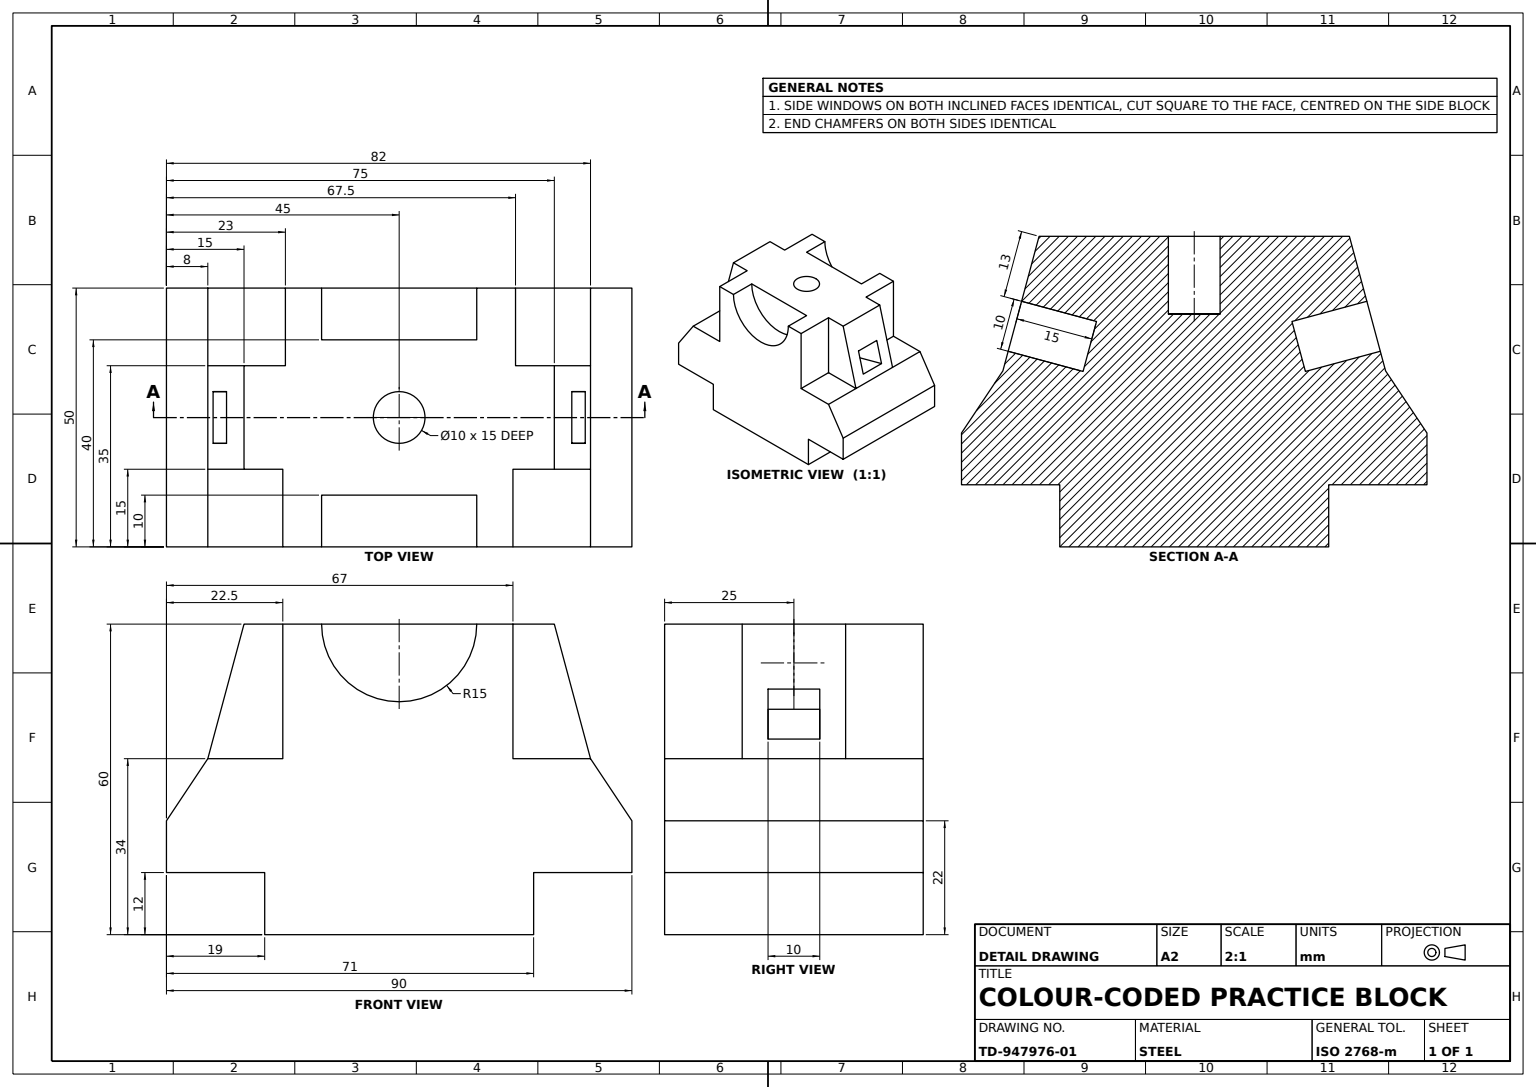
SolidWorks part; units mm, degrees
material "Plain Carbon Steel"
ref_plane "Front Plane" through (0, 0, 0) normal (0, 0, 1) x (1, 0, 0)
ref_plane "Top Plane" through (0, 0, 0) normal (0, 1, 0) x (1, 0, 0)
ref_plane "Right Plane" through (0, 0, 0) normal (1, 0, 0) x (0, 0, -1)
sketch "Base Profile Sketch" plane through (0, 0, 0) normal (0, 0, 1) x (1, 0, 0)
  line L0 (0, 0) -> (52, 0)
  line L1 (52, 0) -> (52, 12)
  line L2 (0, 0) -> (0, 12)
  line L3 (0, 12) -> (-19, 12)
  line L4 (-19, 12) -> (-19, 22)
  line L5 (52, 12) -> (71, 12)
  line L6 (71, 12) -> (71, 22)
  line L7 (4, 34) -> (-11, 34)
  line L8 (-11, 34) -> (-19, 22)
  line L9 (48, 34) -> (63, 34)
  line L10 (48, 34) -> (48, 60)
  line L11 (4, 34) -> (4, 60)
  line L12 (63, 34) -> (71, 22)
  line L13 (4, 60) -> (48, 60)
  dimension "D1" = 8
  dimension "D2" = 19
  dimension "D3" = 23
  dimension "D4" = 67
  dimension "D5" = 12
  dimension "D6" = 22
  dimension "D7" = 34
  dimension "D8" = 60
extrude "Base Block" add sketch "Base Profile Sketch" along normal blind 50
sketch "Saddle Cut 1 Sketch" plane through (0, 0, 50) normal (0, 0, 1) x (1, 0, 0)
  line L0 (48, 60) -> (4, 60) construction
  line L1 (11, 60) -> (41, 60)
  arc A0 (11, 60) -> (41, 60) centre (26, 60) ccw
  dimension "D1" = 30
  dimension "D2" = 15
extrude "Saddle Cut 1 Ø30" cut sketch "Saddle Cut 1 Sketch" against normal blind 10
sketch "Saddle Cut 2 Sketch" plane through (0, 0, 0) normal (0, 0, -1) x (-1, 0, 0)
  line L0 (-48, 60) -> (-4, 60) construction
  line L1 (-41, 60) -> (-11, 60)
  arc A0 (-41, 60) -> (-11, 60) centre (-26, 60) ccw
  dimension "D1" = 30
  dimension "D2" = 15
extrude "Saddle Cut 2 Ø30" cut sketch "Saddle Cut 2 Sketch" against normal blind 10
sketch "Upper Block Sketch" plane through (0, 0, 0) normal (0, 0, -1) x (-1, 0, 0)
  line L0 (-48, 60) -> (-48, 34)
  line L1 (-48, 34) -> (-63, 34)
  line L2 (-48, 60) -> (-56, 60)
  line L3 (-56, 60) -> (-63, 34)
  line L4 (-71, 12) -> (-71, 22) construction
  dimension "D1" = 15
extrude "Upper Block" add sketch "Upper Block Sketch" against normal blind 30
sketch "Upper Block Notch Sketch" plane through (0, 0, 0) normal (0, 0, -1) x (-1, 0, 0)
  line L0 (-63, 34) -> (-56, 60)
  line L1 (-56, 60) -> (-48.5, 60)
  line L2 (0, 12) -> (0, 0) construction
  line L3 (-48.5, 60) -> (-48.5, 34)
  line L4 (-48.5, 34) -> (-63, 34)
  dimension "D1" = 48.5
extrude "Upper Block Notch" cut sketch "Upper Block Notch Sketch" against normal blind 20
sketch "Notch Pad 1 Sketch" plane through (0, 0, 20) normal (0, 0, -1) x (-1, 0, 0)
  line L0 (-63, 34) -> (-48.5, 34)
  line L1 (-48.5, 34) -> (-48.5, 60)
  line L2 (-48.5, 60) -> (-56, 60)
  line L3 (-56, 60) -> (-63, 34)
extrude "Notch Pad 1" add sketch "Notch Pad 1 Sketch" along normal blind 5
sketch "Notch Pad 2 Sketch" plane through (0, 0, 30) normal (0, 0, 1) x (1, 0, 0)
  line L0 (48, 60) -> (56, 60)
  line L1 (56, 60) -> (63, 34)
  line L2 (63, 34) -> (48, 34)
  line L3 (48, 34) -> (48, 60)
extrude "Notch Pad 2" add sketch "Notch Pad 2 Sketch" along normal blind 5
sketch "Side Block Sketch" plane through (0, 0, 50) normal (0, 0, 1) x (1, 0, 0)
  line L0 (4, 60) -> (4, 34)
  line L1 (4, 34) -> (-11, 34)
  line L2 (4, 60) -> (-4, 60)
  line L3 (-4, 60) -> (-11, 34)
  line L4 (-19, 22) -> (-19, 12) construction
  dimension "D1" = 15
extrude "Side Block" add sketch "Side Block Sketch" against normal blind 35
sketch "Side Block Pocket Sketch" plane through (0, 0, 50) normal (0, 0, 1) x (1, 0, 0)
  line L2 (11, 60) -> (-4, 60) construction
  line L3 (3.5, 60) -> (3.5, 34)
  line L4 (3.5, 34) -> (-11, 34)
  line L5 (-11, 34) -> (-4, 60)
  line L6 (-4, 60) -> (3.5, 60)
extrude "Side Block Pocket" cut sketch "Side Block Pocket Sketch" against normal blind 15
sketch "Top Hole Sketch" plane through (0, 60, 0) normal (0, 1, 0) x (1, 0, 0)
  line L0 (56, -35) -> (56, -15) construction
  line L1 (41, -40) -> (11, -40) construction
  circle A1 centre (26, -25) radius 5
  dimension "D1" = 10
  dimension "D2" = 10
  dimension "D3" = 30
  dimension "D4" = 15
extrude "Top Hole Ø10" cut sketch "Top Hole Sketch" against normal blind 15
sketch "Side Window Sketch" plane through (-18.7917, 5.0593, 0) normal (-0.9656, 0.26, 0) x (0, 0, 1)
  line L0 (35, 56.8971) -> (35, 29.9712) construction
  line L1 (20, 43.8971) -> (30, 43.8971)
  line L2 (20, 43.8971) -> (20, 33.8971)
  line L3 (20, 33.8971) -> (30, 33.8971)
  line L4 (30, 43.8971) -> (30, 33.8971)
  line L6 (15, 56.8971) -> (35, 56.8971) construction
  dimension "D1" = 5
  dimension "D2" = 13
  dimension "D3" = 5
extrude "Side Window Cut" cut sketch "Side Window Sketch" against normal blind 15
sketch "Upper Window Sketch" plane through (67.2772, 18.1131, 0) normal (0.9656, 0.26, 0) x (0, 0, -1)
  line L0 (-35, 16.4526) -> (-35, 43.3784) construction
  line L1 (-30, 30.3784) -> (-20, 30.3784)
  line L2 (-30, 30.3784) -> (-30, 20.3784)
  line L3 (-30, 20.3784) -> (-20, 20.3784)
  line L4 (-20, 30.3784) -> (-20, 20.3784)
  line L5 (-15, 43.3784) -> (-15, 16.4526) construction
  line L6 (-35, 43.3784) -> (-15, 43.3784) construction
  dimension "D1" = 5
  dimension "D2" = 5
  dimension "D3" = 13
extrude "Upper Window Cut" cut sketch "Upper Window Sketch" against normal blind 15
